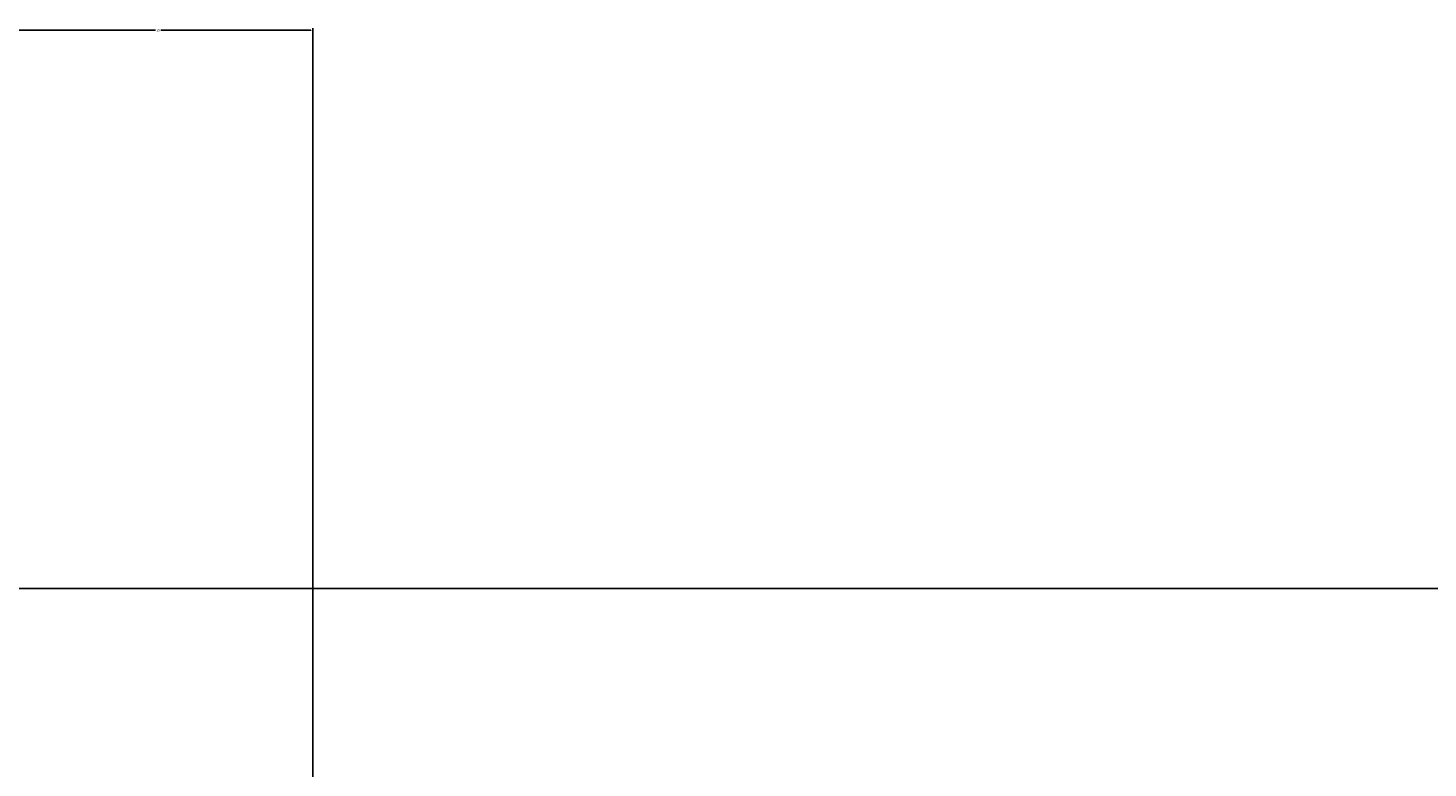
# Model space of a CAD drawing. Units: feet. Extents: x 105 to 1094, y -88 to 588.
# Tile 58 of 59: x 649 to 762, y 529 to 588. Entities that reach past the tile are written whole.
import ezdxf

# ---------------------------------------------------------------- set-up
doc = ezdxf.new("R2010")
doc.units = ezdxf.units.FT
doc.header["$MEASUREMENT"] = 0
doc.layers.add('A-ANNO-DIMS', color=2, linetype='Continuous', lineweight=18)
doc.styles.get("Standard").update_dxf_attribs({"font": 'arial.ttf'})
doc.dimstyles.get("Standard").update_dxf_attribs({"dimtxt": 0.18, "dimasz": 0.18, "dimexe": 0.18, "dimexo": 0.0625, "dimgap": 0.09, "dimtad": 0, "dimtih": 1, "dimtoh": 1, "dimdec": 4, "dimzin": 0, "dimdsep": 46, "dimtxsty": 'Standard', "dimcen": 0.09, "dimadec": 0, "dimazin": 0, "dimtfac": 1, "dimtdec": 4, "dimtofl": 0, "dimtmove": 0, "dimatfit": 3, "dimfxl": 1, "dimtolj": 1, "dimtzin": 0, "dimarcsym": 0})

# ---------------------------------------------------------------- blocks, each defined once
blk = doc.blocks.new('*D21')
at = {"layer": 'A-ANNO-DIMS', "color": 0, "lineweight": -2, "transparency": 16777216}
for p, q in [((849.63, 543.08), (105.46, 543.08)), ((105.64, 542.9), (105.64, 250.26)), ((105.64, -42.74), (105.64, 249.9)), ((849.63, -42.92), (105.46, -42.92))]:
    blk.add_line(p, q, dxfattribs=at)
at = {"layer": 'A-ANNO-DIMS', "color": 0, "transparency": 16777216}
for points in [[(105.61, 542.9), (105.67, 542.9), (105.64, 543.08)], [(105.61, -42.74), (105.67, -42.74), (105.64, -42.92)]]:
    blk.add_solid(points, dxfattribs=at)
at = {"layer": 'Defpoints', "color": 0, "transparency": 16777216}
for p in [(105.64, 543.08), (849.69, 543.08), (849.69, -42.92)]:
    blk.add_point(p, dxfattribs=at)
at = {"layer": 'A-ANNO-DIMS', "color": 0, "transparency": 16777216, "insert": (105.64, 250.08), "char_height": 0.18, "attachment_point": 5}
blk.add_mtext('\\A1;586', dxfattribs=at)
blk = doc.blocks.new('*D30')
at = {"layer": 'A-ANNO-DIMS', "color": 0, "lineweight": -2, "transparency": 16777216}
for p, q in [((349.75, 543.08), (1093.92, 543.08)), ((1093.74, 542.9), (1093.74, 535.26)), ((1093.74, 527.26), (1093.74, 534.9)), ((349.75, 527.08), (1093.92, 527.08))]:
    blk.add_line(p, q, dxfattribs=at)
at = {"layer": 'A-ANNO-DIMS', "color": 0, "transparency": 16777216}
for points in [[(1093.71, 542.9), (1093.77, 542.9), (1093.74, 543.08)], [(1093.71, 527.26), (1093.77, 527.26), (1093.74, 527.08)]]:
    blk.add_solid(points, dxfattribs=at)
at = {"layer": 'Defpoints', "color": 0, "transparency": 16777216}
for p in [(349.69, 543.08), (349.69, 527.08), (1093.74, 527.08)]:
    blk.add_point(p, dxfattribs=at)
at = {"layer": 'A-ANNO-DIMS', "color": 0, "transparency": 16777216, "insert": (1093.74, 535.08), "char_height": 0.18, "attachment_point": 5}
blk.add_mtext('\\A1;16', dxfattribs=at)
blk = doc.blocks.new('*D41')
at = {"layer": 'A-ANNO-DIMS', "color": 0, "lineweight": -2, "transparency": 16777216}
for p, q in [((646.69, 441.14), (646.69, 588.31)), ((646.87, 588.13), (658.97, 588.13)), ((671.51, 588.13), (659.41, 588.13)), ((671.69, 441.14), (671.69, 588.31))]:
    blk.add_line(p, q, dxfattribs=at)
at = {"layer": 'A-ANNO-DIMS', "color": 0, "transparency": 16777216}
for points in [[(646.87, 588.16), (646.87, 588.1), (646.69, 588.13)], [(671.51, 588.16), (671.51, 588.1), (671.69, 588.13)]]:
    blk.add_solid(points, dxfattribs=at)
at = {"layer": 'Defpoints', "color": 0, "transparency": 16777216}
for p in [(671.69, 588.13), (646.69, 441.08), (671.69, 441.08)]:
    blk.add_point(p, dxfattribs=at)
at = {"layer": 'A-ANNO-DIMS', "color": 0, "transparency": 16777216, "insert": (659.19, 588.13), "char_height": 0.18, "attachment_point": 5}
blk.add_mtext('\\A1;25', dxfattribs=at)

msp = doc.modelspace()

# ---------------------------------------------------------------- dimensions: what is measured, and where the dimension line sits
at = {"layer": 'A-ANNO-DIMS'}
dim = msp.add_linear_dim(base=(671.6883, 588.1312), p1=(646.6883, 441.0812), p2=(671.6883, 441.0812), dimstyle='Standard', override={"dimdec": 0, "dimlfac": 1, "dimrnd": 0, "dimzin": 0, "dimdsep": 46, "dimlunit": 2}, dxfattribs=at)
dim.commit()
dim.dimension.update_dxf_attribs({"geometry": '*D41', "text_midpoint": (659.1883, 588.1312)})
for base, p1, p2, picture, middle in [((105.6383, 543.0812), (849.6883, -42.9188), (849.6883, 543.0812), '*D21', (105.6383, 250.0812)), ((1093.7383, 527.0812), (349.6883, 543.0812), (349.6883, 527.0812), '*D30', (1093.7383, 535.0812))]:
    dim = msp.add_linear_dim(base=base, p1=p1, p2=p2, angle=90, dimstyle='Standard', override={"dimdec": 0, "dimlfac": 1, "dimrnd": 0, "dimzin": 0, "dimdsep": 46, "dimlunit": 2}, dxfattribs=at)
    dim.commit()
    dim.dimension.update_dxf_attribs({"geometry": picture, "text_midpoint": middle})

doc.saveas('drawing.dxf')
